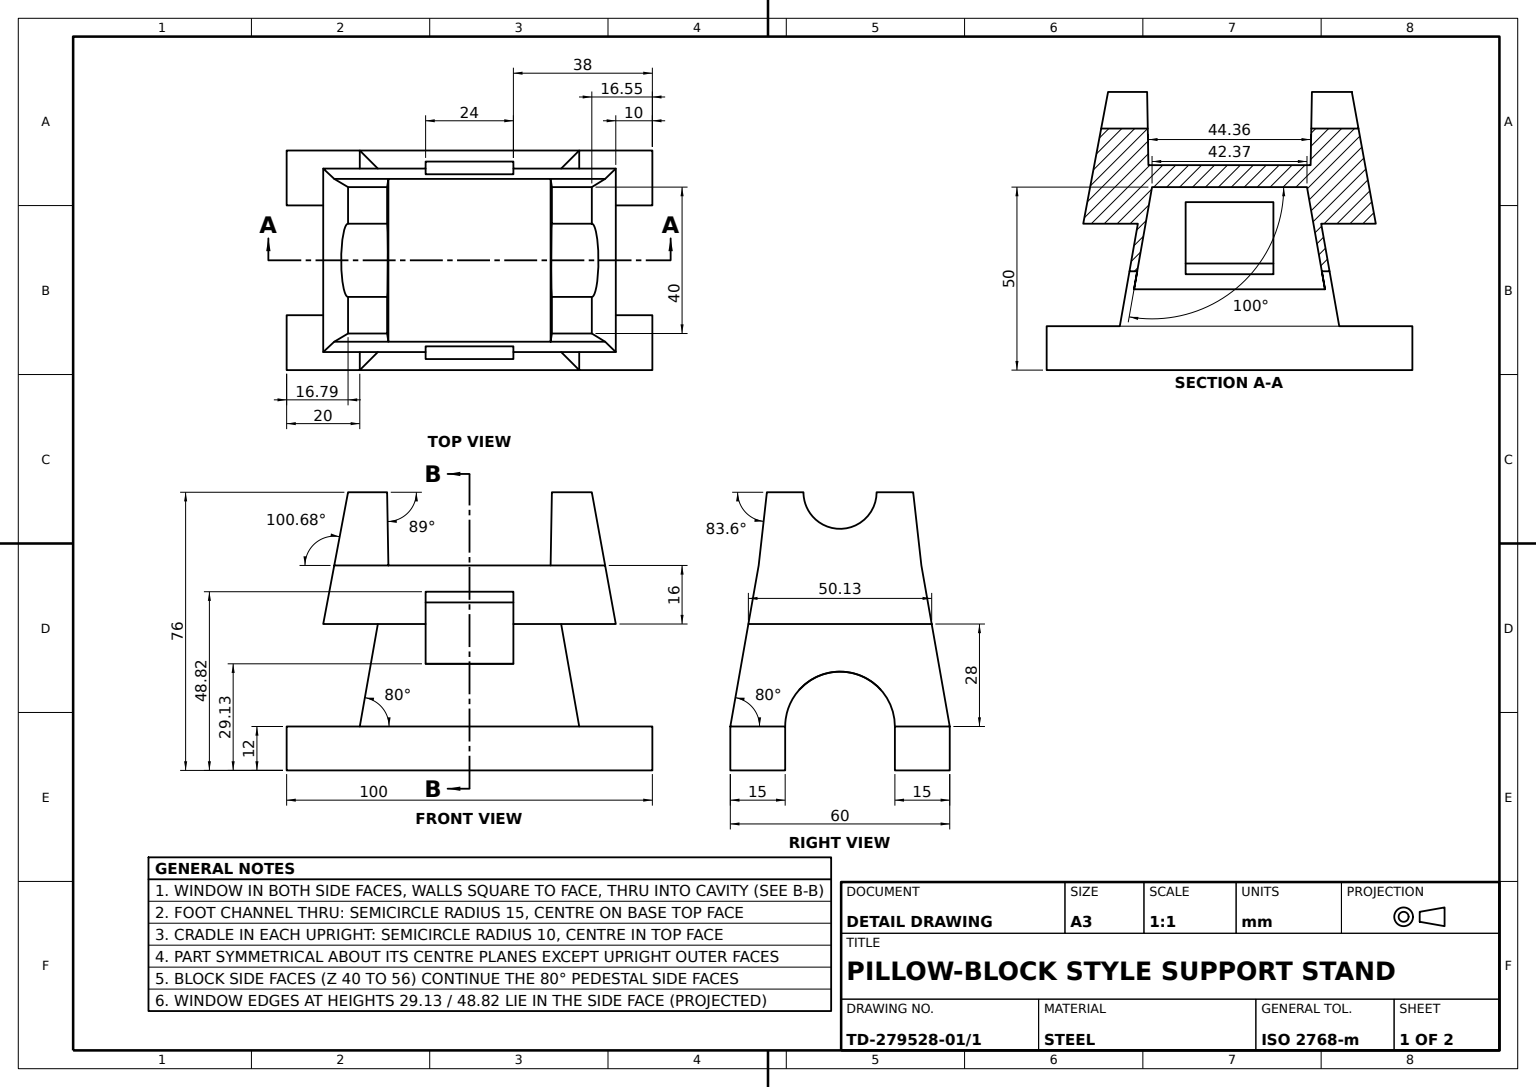
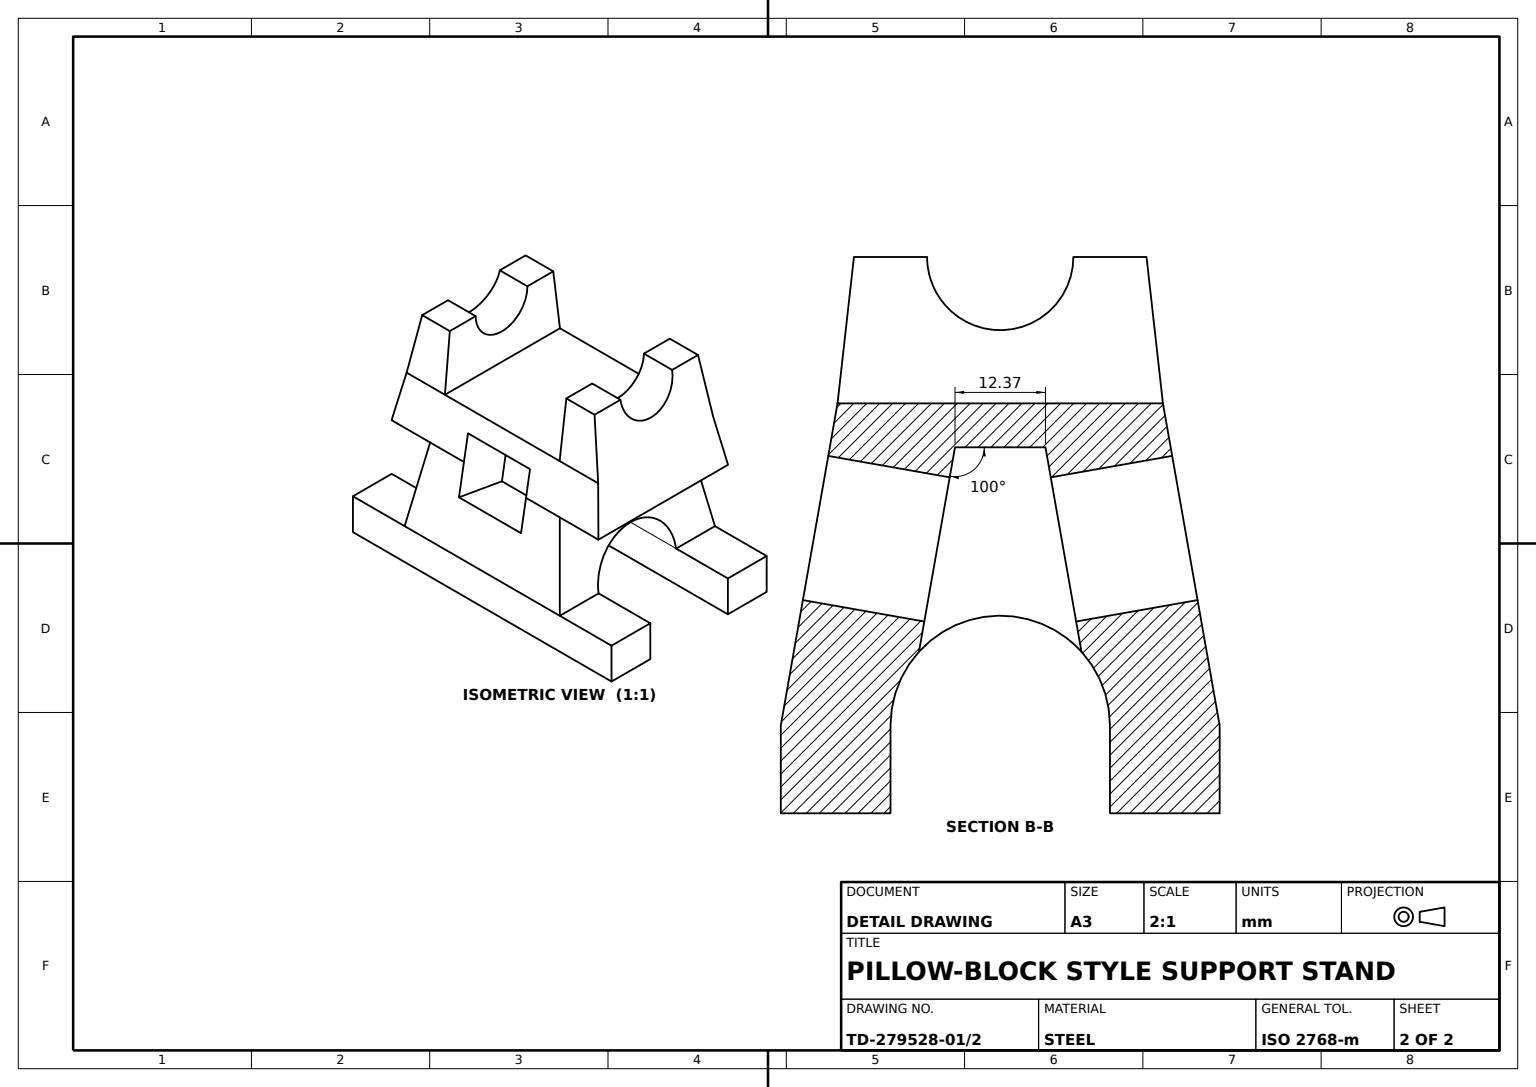
SolidWorks part; units mm, degrees
material "Plain Carbon Steel"
ref_plane "Front Plane" through (0, 0, 0) normal (0, 0, 1) x (1, 0, 0)
ref_plane "Top Plane" through (0, 0, 0) normal (0, 1, 0) x (1, 0, 0)
ref_plane "Right Plane" through (0, 0, 0) normal (1, 0, 0) x (0, 0, -1)
sketch "Base Plate Sketch" plane through (0, 0, 0) normal (0, 1, 0) x (1, 0, 0)
  line L1 (-30, -50) -> (30, -50)
  line L2 (-30, -50) -> (-30, 50)
  line L3 (-30, 50) -> (30, 50)
  line L4 (30, -50) -> (30, 50)
  line L5 (-30, -50) -> (30, 50) construction
  line L6 (-30, 50) -> (30, -50) construction
  point P0 (0, 0)
  dimension "D1" = 100
  dimension "D2" = 60
extrude "Base Plate 100x60x12" add sketch "Base Plate Sketch" along normal blind 12
sketch "Pedestal Sketch" plane through (0, 12, 0) normal (0, 1, 0) x (1, 0, 0)
  line L0 (30, -50) -> (30, 50) construction
  line L1 (-30, 30) -> (30, 30)
  line L2 (-30, 30) -> (-30, -30)
  line L3 (-30, -30) -> (30, -30)
  line L4 (30, 30) -> (30, -30)
  line L5 (-30, 30) -> (30, -30) construction
  line L6 (-30, -30) -> (30, 30) construction
  point P0 (0, 0)
extrude "Tapered Pedestal" add sketch "Pedestal Sketch" along normal blind 28 draft 10
sketch "Foot Channel Sketch" plane through (0, 0, 50) normal (0, 0, 1) x (1, 0, 0)
  line L0 (-15, 0) -> (15, 0)
  line L1 (-30, 0) -> (30, 0) construction
  line L2 (-15, 0) -> (-15, 12)
  line L3 (-30, 12) -> (30, 12) construction
  line L4 (-15, 12) -> (15, 12)
  line L5 (15, 12) -> (15, 0)
  arc A0 (-15, 12) -> (15, 12) centre (0, 12) cw
  point P6 (0, 0)
  line M1 (-30, 0) -> (30, 0)
  line M3 (30, 12) -> (-30, 12)
  dimension "D1" = 15
extrude "Foot Channel Cut" cut sketch "Foot Channel Sketch" against normal blind 200 contours A0 M3 | L5 L2 M3 M1
sketch "Upper Block Sketch" plane through (0, 40, 0) normal (0, 1, 0) x (1, 0, 0)
  line L1 (-25.065, 40) -> (25.065, 40)
  line L2 (-25.065, 40) -> (-25.065, -40)
  line L3 (-25.065, -40) -> (25.065, -40)
  line L4 (25.065, 40) -> (25.065, -40)
  line L5 (-25.065, 40) -> (25.065, -40) construction
  line L6 (-25.065, -40) -> (25.065, 40) construction
  point P0 (0, 0)
  dimension "D1" = 80
  dimension "D2" = 50.13
extrude "Upper Block 80x50" add sketch "Upper Block Sketch" along normal blind 16 draft 10
sketch "Top Slot Sketch" plane through (31.1496, 5.4925, 0) normal (0.9848, 0.1736, 0) x (0, 0, -1)
  line L0 (0, 0) -> (0, 24)
  line L1 (-12, 24) -> (12, 24)
  line L2 (-40, 35.0398) -> (40, 35.0398) construction
  line L3 (-12, 24) -> (12, 24)
  line L4 (-12, 24) -> (-12, 44)
  line L5 (-12, 44) -> (12, 44)
  line L6 (12, 24) -> (12, 44)
  point P6 (0, 24)
  line M4 (-40, 35.0398) -> (40, 35.0398)
  dimension "D1" = 24
  dimension "D2" = 20
  dimension "D3" = 24
  dimension "D4" = 28
  dimension "D5" = 40
  dimension "D6" = 8.9602
extrude "Top Slot Cut" cut sketch "Top Slot Sketch" against normal blind 16 contours L6 L5 L4 M4 | L1 L6 L4 M4
sketch "Pedestal Relief Sketch" plane through (0, 0, 0) normal (0, -1, 0) x (1, 0, 0)
  line L0 (15, 50) -> (15, -50) construction
  line L1 (-15, 30) -> (15, 30)
  line L2 (-15, 30) -> (-15, -30)
  line L3 (-15, -30) -> (15, -30)
  line L4 (15, 30) -> (15, -30)
  line L5 (15, -30) -> (15, 30) construction
  dimension "D1" = 60
extrude "Pedestal Relief Cut" cut sketch "Pedestal Relief Sketch" against normal blind 50 draft 10
sketch "Window Sketch" plane through (15.3927, 2.7141, 0) normal (0.9848, 0.1736, 0) x (0, 0, -1)
  line L0 (12, 24) -> (12, 44) construction
  line L1 (-12, 44) -> (12, 44)
  line L2 (-12, 44) -> (-12, 24)
  line L3 (-12, 24) -> (12, 24)
  line L4 (12, 44) -> (12, 24)
  dimension "D1" = 20
extrude "Square Window 20x20" cut sketch "Window Sketch" against normal blind 5
sketch "Side Pocket Sketch" plane through (-31.1496, 5.4925, 0) normal (-0.9848, 0.1736, 0) x (0, 0, 1)
  line L0 (-40, 35.0398) -> (40, 35.0398) construction
  line L1 (-12, 24) -> (12, 24)
  line L3 (-12, 24) -> (12, 24)
  line L4 (-12, 24) -> (-12, 44)
  line L5 (-12, 44) -> (12, 44)
  line L6 (12, 24) -> (12, 44)
  point P6 (0, 24)
  line M5 (-40, 35.0398) -> (40, 35.0398)
  dimension "D1" = 28
  dimension "D2" = 24
  dimension "D3" = 20
  dimension "D4" = 8.9602
extrude "Side Pocket Cut" cut sketch "Side Pocket Sketch" against normal blind 20 contours L6 L5 L4 M5 | L1 L6 L4 M5
sketch "Rib Boss Sketch" plane through (0, 56, 0) normal (0, 1, 0) x (1, 0, 0)
  line L1 (-22.2438, 37.1788) -> (22.2438, 37.1788)
  line L2 (-22.2438, 37.1788) -> (-22.2438, -37.1788)
  line L3 (-22.2438, -37.1788) -> (22.2438, -37.1788)
  line L4 (22.2438, 37.1788) -> (22.2438, -37.1788)
extrude "Rib Boss" add sketch "Rib Boss Sketch" along normal blind 20 draft 10
sketch "Trim Sketch" plane through (0, 0, 50) normal (0, 0, 1) x (1, 0, 0)
  line L0 (-15, 0) -> (-15, 12) construction
  line L1 (-30, 12) -> (-15, 12) construction
  line L2 (0, 56) -> (24.9625, 56)
  line L3 (24.9625, 56) -> (24.9625, 76)
  line L4 (24.9625, 76) -> (-29.1618, 76)
  line L5 (-29.1618, 76) -> (-29.1618, 56)
  line L6 (-29.1618, 56) -> (0, 56)
  point P3 (0, 47.1914)
  dimension "D1" = 15
  dimension "D2" = 39.9625
  dimension "D3" = 14.1618
  dimension "D4" = 35.1914
  dimension "D5" = 44
  dimension "D6" = 64
extrude "Trim Cut" cut sketch "Trim Sketch" against normal blind 100
sketch "Uprights Sketch" plane through (0, 56, 0) normal (0, 1, 0) x (1, 0, 0)
  line L0 (22.2438, 37.1788) -> (22.2438, -37.1788) construction
  line L1 (-22.2438, 37.1788) -> (22.2438, 37.1788)
  line L2 (-22.2438, 37.1788) -> (-22.2438, 22.1788)
  line L3 (-22.2438, 22.1788) -> (22.2438, 22.1788)
  line L4 (22.2438, 37.1788) -> (22.2438, 22.1788)
  line L6 (-22.2438, -37.1788) -> (22.2438, -37.1788)
  line L7 (-22.2438, -37.1788) -> (-22.2438, -22.1788)
  line L8 (-22.2438, -22.1788) -> (22.2438, -22.1788)
  line L9 (22.2438, -37.1788) -> (22.2438, -22.1788)
  dimension "D1" = 15
  dimension "D2" = 15
extrude "Uprights 15x15" add sketch "Uprights Sketch" along normal blind 20 draft 1
sketch "Cradle Cut A Sketch" plane through (0, 0, 50) normal (0, 0, 1) x (1, 0, 0)
  line L0 (-15, 0) -> (-15, 12) construction
  line L1 (-21.8947, 76) -> (21.8947, 76) construction
  line L3 (20, 76) -> (22.2438, 56)
  line L5 (-22.2438, 56) -> (-20, 76)
  line L6 (20, 76) -> (21.8947, 76)
  line L7 (21.8947, 76) -> (22.2438, 56)
  line L8 (-20, 76) -> (-21.8947, 76)
  line L9 (-21.8947, 76) -> (-22.2438, 56)
  dimension "D1" = 35
extrude "Cradle Cut A" cut sketch "Cradle Cut A Sketch" against normal blind 200
sketch "Cradle Cut B Sketch" plane through (30, 0, 0) normal (1, 0, 0) x (0, 0, -1)
  line L0 (-40, 40) -> (-33.2082, 76)
  line L1 (-36.8297, 76) -> (-22.5279, 76) construction
  line L2 (-33.2082, 76) -> (-36.8297, 76)
  line L3 (-36.8297, 76) -> (-40, 40)
  line L4 (40, 40) -> (33.4454, 76)
  line L5 (36.8297, 76) -> (22.5279, 76) construction
  line L6 (33.4454, 76) -> (36.8297, 76)
  line L7 (36.8297, 76) -> (40, 40)
  dimension "D1" = 3.4454
  dimension "D2" = 63.2082
extrude "Cradle Cut B" cut sketch "Cradle Cut B Sketch" against normal blind 200
sketch "Cross Bore Sketch" plane through (0, 0, 50) normal (0, 0, 1) x (1, 0, 0)
  line L0 (-20, 76) -> (20, 76) construction
  line L1 (-10, 76) -> (10, 76)
  arc A0 (-10, 76) -> (10, 76) centre (0, 76) ccw
  dimension "D1" = 10
extrude "Cross Bore Cut" cut sketch "Cross Bore Sketch" against normal blind 100
